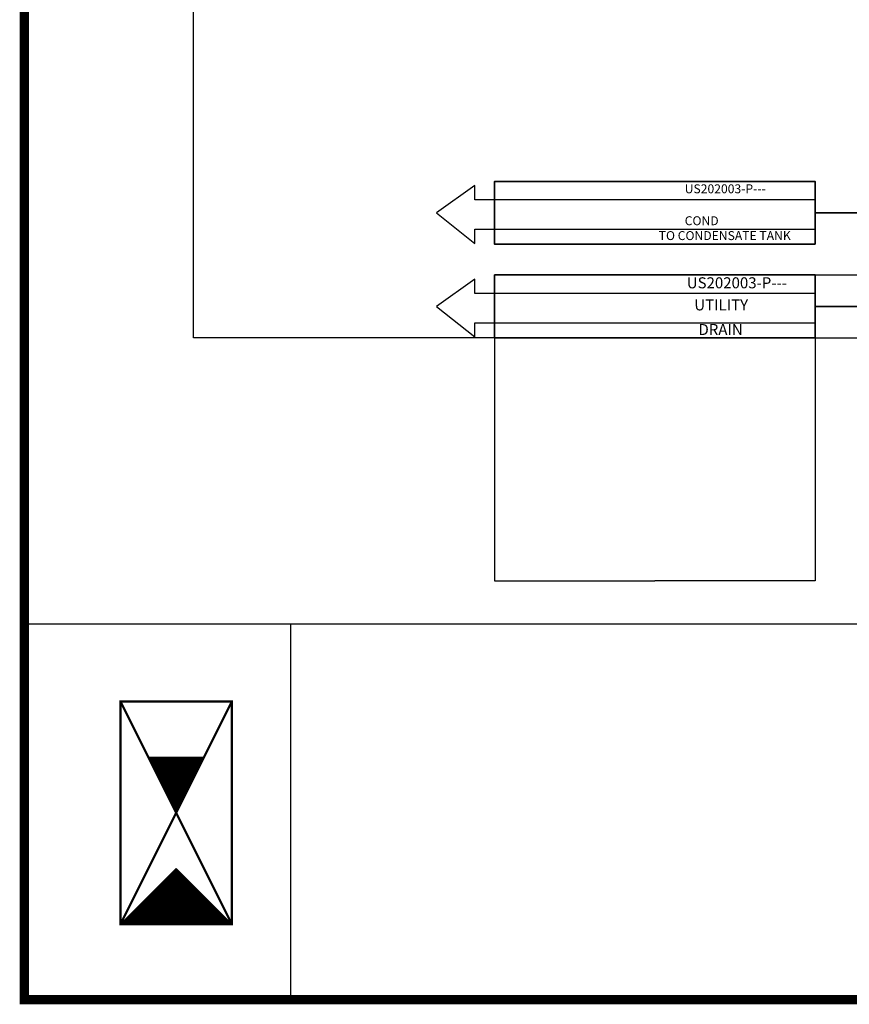
# Model space of a CAD drawing. Units: millimetres. Extents: x 353872 to 441597, y 126154 to 187356.
# Tile 1 of 28: x 353872 to 367541, y 126840 to 143050. Entities that reach past the tile are written whole.
import ezdxf

# ---------------------------------------------------------------- set-up
doc = ezdxf.new("R2010")
doc.units = ezdxf.units.MM
for name, color, linetype, lineweight in [('.', 7, 'Continuous', 0), ('A-ANNO-DIMS', 2, 'Continuous', 18), ('P-ANNO-TEXT', 7, 'Continuous', 25), ('P-ANNO-TTLB', 7, 'Continuous', 25), ('P-EQPM', 5, 'Continuous', 35), ('P-PIPE', 3, 'Continuous', 35)]:
    doc.layers.add(name, color=color, linetype=linetype, lineweight=lineweight)
doc.styles.get("Standard").update_dxf_attribs({"font": 'arial.ttf'})
doc.dimstyles.get("Standard").update_dxf_attribs({"dimtxt": 0.18, "dimasz": 0.18, "dimexe": 0.18, "dimexo": 0.0625, "dimgap": 0.09, "dimtad": 0, "dimtih": 1, "dimtoh": 1, "dimdec": 4, "dimzin": 0, "dimdsep": 46, "dimtxsty": 'Standard', "dimcen": 0.09, "dimadec": 0, "dimazin": 0, "dimtfac": 1, "dimtdec": 4, "dimtofl": 0, "dimtmove": 0, "dimatfit": 3, "dimfxl": 1, "dimtolj": 1, "dimtzin": 0, "dimarcsym": 0})
pattern_1 = [(45, (0, 0), (-0.0883883476483185, 0.0883883476483185), [])]

# ---------------------------------------------------------------- blocks, each defined once
blk = doc.blocks.new('LOGO')
at = {"layer": '.', "ltscale": 0.5}
h = blk.add_hatch(dxfattribs=at)
h.set_pattern_fill('ANSI31', color=256)
h.set_pattern_definition(pattern_1)
h.paths.add_polyline_path([(-25, 50), (0, 0), (25, 50)])
h = blk.add_hatch(dxfattribs=at)
h.set_pattern_fill('ANSI31', color=256)
h.set_pattern_definition(pattern_1)
h.paths.add_polyline_path([(50, -100), (-1.8e-15, -49.99999999906868), (-50, -100)])
at = {"ltscale": 0.5}
blk.add_line((-25, 50), (25, 50), dxfattribs=at)
at = {"ltscale": 0.5, "const_width": 2}
for points in [[(-50, 100), (-50, 100), (0, 0), (50, 100), (50, 100)], [(-50, -100), (-50, -100), (0, 0), (50, -100), (50, -100)]]:
    blk.add_lwpolyline(points, dxfattribs=at)
blk.add_lwpolyline([(-50, 100), (50, 100), (50, -100), (-50, -100)], close=True, dxfattribs=at)
at = {"ltscale": 0.5}
blk.add_lwpolyline([(-50, -100), (0, -49.99999999906868), (50, -100), (-50, -100)], dxfattribs=at)
blk = doc.blocks.new('*D25')
at = {"layer": 'A-ANNO-DIMS', "color": 0, "lineweight": -2, "transparency": 16777216}
for p, q in [((360736.4843020002, 182546.052974), (356736.3668020003, 182546.052974)), ((356736.5468020003, 182545.8729740001), (356736.5468020003, 160179.6269640294)), ((356736.5468020003, 137813.017025), (356736.5468020003, 160179.2630349707)), ((361695.7183060002, 137812.837025), (356736.3668020003, 137812.837025))]:
    blk.add_line(p, q, dxfattribs=at)
at = {"layer": 'A-ANNO-DIMS', "color": 0, "transparency": 16777216}
for points in [[(356736.5168020002, 182545.8729740001), (356736.5768020003, 182545.8729740001), (356736.5468020003, 182546.052974)], [(356736.5168020002, 137813.017025), (356736.5768020003, 137813.017025), (356736.5468020003, 137812.837025)]]:
    blk.add_solid(points, dxfattribs=at)
at = {"layer": 'Defpoints', "color": 0, "transparency": 16777216}
for p in [(360736.5468020002, 182546.052974), (356736.5468020003, 137812.837025), (361695.7808060001, 137812.837025)]:
    blk.add_point(p, dxfattribs=at)
at = {"layer": 'A-ANNO-DIMS', "color": 0, "transparency": 16777216, "insert": (356736.5468020003, 160179.4449994999), "char_height": 0.18, "attachment_point": 5}
blk.add_mtext('\\A1;44733', dxfattribs=at)
blk = doc.blocks.new('*D26')
at = {"layer": 'A-ANNO-DIMS', "color": 0, "lineweight": -2, "transparency": 16777216}
for p, q in [((361695.780806, 137812.774525), (361695.780806, 133812.657025)), ((366976.7551870001, 137812.774525), (366976.7551870001, 133812.657025)), ((361695.960806, 133812.837025), (364335.9265981371, 133812.837025)), ((366976.575187, 133812.837025), (364336.609394863, 133812.837025))]:
    blk.add_line(p, q, dxfattribs=at)
at = {"layer": 'A-ANNO-DIMS', "color": 0, "transparency": 16777216}
for points in [[(361695.960806, 133812.867025), (361695.960806, 133812.807025), (361695.780806, 133812.837025)], [(366976.575187, 133812.867025), (366976.575187, 133812.807025), (366976.7551870001, 133812.837025)]]:
    blk.add_solid(points, dxfattribs=at)
at = {"layer": 'Defpoints', "color": 0, "transparency": 16777216}
for p in [(361695.780806, 137812.837025), (366976.7551870001, 137812.837025), (366976.7551870001, 133812.837025)]:
    blk.add_point(p, dxfattribs=at)
at = {"layer": 'A-ANNO-DIMS', "color": 0, "transparency": 16777216, "insert": (364336.2679965, 133812.837025), "char_height": 0.18, "attachment_point": 5}
blk.add_mtext('\\A1;5281', dxfattribs=at)
blk = doc.blocks.new('*D27')
at = {"layer": 'A-ANNO-DIMS', "color": 0, "lineweight": -2, "transparency": 16777216}
for p, q in [((366976.8176870001, 138848.060561), (440591.1818100004, 138848.060561)), ((440591.0018100004, 138847.8805610001), (440591.0018100004, 138330.6307575294)), ((440591.0018100004, 137813.017025), (440591.0018100004, 138330.2668284707)), ((366976.8176870001, 137812.837025), (440591.1818100004, 137812.837025))]:
    blk.add_line(p, q, dxfattribs=at)
at = {"layer": 'A-ANNO-DIMS', "color": 0, "transparency": 16777216}
for points in [[(440590.9718100004, 138847.8805610001), (440591.0318100004, 138847.8805610001), (440591.0018100004, 138848.060561)], [(440590.9718100004, 137813.017025), (440591.0318100004, 137813.017025), (440591.0018100004, 137812.837025)]]:
    blk.add_solid(points, dxfattribs=at)
at = {"layer": 'Defpoints', "color": 0, "transparency": 16777216}
for p in [(366976.7551870001, 138848.060561), (366976.7551870001, 137812.837025), (440591.0018100004, 137812.837025)]:
    blk.add_point(p, dxfattribs=at)
at = {"layer": 'A-ANNO-DIMS', "color": 0, "transparency": 16777216, "insert": (440591.0018100004, 138330.4487929999), "char_height": 0.18, "attachment_point": 5}
blk.add_mtext('\\A1;1035.2', dxfattribs=at)

msp = doc.modelspace()

# ---------------------------------------------------------------- linework, layer by layer
at = {"layer": 'P-ANNO-TTLB'}
msp.add_line((353948.027365095, 133103.9219526489), (440835.1896390488, 133103.9219526489), dxfattribs=at)
at = {"layer": 'P-ANNO-TTLB', "ltscale": 0.5}
msp.add_line((358335.0178812332, 133103.9219526489), (358335.0178812332, 126916.340154238), dxfattribs=at)
at = {"layer": 'P-ANNO-TTLB', "const_width": 152.4336180244531}
msp.add_lwpolyline([(353948.027365095, 187280.0528919451), (353948.027365095, 126916.340154238), (440835.1896390488, 126916.340154238), (440835.1896390488, 187280.0528919451)], close=True, dxfattribs=at)
at = {"layer": 'P-ANNO-TTLB'}
for points in [[(366976.7551871072, 140084.5530813161), (361369.9490425979, 140084.5530813161), (361369.9490425979, 140318.5333806309), (360736.5468018789, 139870.4641427255), (361369.9490425979, 139367.4195692754), (361369.9490425979, 139601.3998685902), (366976.7551871072, 139601.3998685902)], [(366976.7551871072, 138544.5377317878), (361369.9490425979, 138544.5377317878), (361369.9490425979, 138778.5180311025), (360736.5468018789, 138330.448793197), (361369.9490425979, 137827.4042197469), (361369.9490425979, 138061.3845190617), (366976.7551871072, 138061.3845190617)]]:
    msp.add_lwpolyline(points, dxfattribs=at)
at = {"layer": 'P-EQPM'}
for points in [[(366976.7551871072, 139352.8523745578), (361695.7808057135, 139352.8523745578), (361695.7808057135, 140388.0759108931), (366976.7551871072, 140388.0759108931)], [(366976.7551871072, 137812.8370250294), (361695.7808057135, 137812.8370250294), (361695.7808057135, 138848.0605613646), (366976.7551871072, 138848.0605613646)]]:
    msp.add_lwpolyline(points, close=True, dxfattribs=at)
at = {"layer": 'P-PIPE'}
msp.add_line((366976.7551871072, 138330.448793197), (381521.2667513259, 138330.448793197), dxfattribs=at)
msp.add_lwpolyline([(378690.5041107035, 139870.4641427255), (378361.7180714816, 139870.4641427255, 0.9912181088121462), (378239.2179874769, 139870.4641427255), (366976.7551871072, 139870.4641427255)], format="xyb", dxfattribs=at)

# ---------------------------------------------------------------- block references
at = {"layer": 'P-ANNO-TTLB', "xscale": 18.34344602605143, "yscale": 18.34344602605143, "zscale": 18.34344602605143}
msp.add_blockref('LOGO', (356450.3617875155, 129992.1658918861), dxfattribs=at)

# ---------------------------------------------------------------- texts
at = {"layer": 'P-ANNO-TEXT'}
for s, height, p in [('US202003-P---', 146.8314391480259, (364828.8239641415, 140192.9325025955)), ('COND', 146.8314391480259, (364828.8239641415, 139667.0009499851)), ('TO CONDENSATE TANK', 146.8314391480259, (364400.0555194523, 139422.383555757)), ('US202003-P---', 181.4449954753344, (364862.7502921565, 138627.9607251264)), ('UTILITY', 181.4449954753344, (364986.4498477008, 138263.9798606744)), ('DRAIN', 181.4449954753344, (365055.2991148313, 137859.1053258672))]:
    msp.add_text(s, height=height, dxfattribs=at).set_placement(p)

# ---------------------------------------------------------------- dimensions: what is measured, and where the dimension line sits
at = {"layer": 'A-ANNO-DIMS'}
for base, p1, p2, override, picture, middle in [((356736.5468020003, 137812.837025), (360736.5468020001, 182546.052974), (361695.780806, 137812.837025), {"dimdec": 0, "dimlfac": 1, "dimrnd": 0, "dimzin": 0, "dimdsep": 46, "dimlunit": 2}, '*D25', (356736.5468020003, 160179.4449994999)), ((440591.0018100004, 137812.837025), (366976.7551870001, 138848.060561), (366976.7551870001, 137812.837025), {"dimdec": 1, "dimlfac": 1, "dimrnd": 0, "dimzin": 0, "dimdsep": 46, "dimlunit": 2}, '*D27', (440591.0018100004, 138330.4487929999))]:
    dim = msp.add_linear_dim(base=base, p1=p1, p2=p2, angle=90, dimstyle='Standard', override=override, dxfattribs=at)
    dim.commit()
    dim.dimension.update_dxf_attribs({"geometry": picture, "text_midpoint": middle})
dim = msp.add_linear_dim(base=(366976.7551870001, 133812.837025), p1=(361695.780806, 137812.837025), p2=(366976.7551870001, 137812.837025), dimstyle='Standard', override={"dimdec": 0, "dimlfac": 1, "dimrnd": 0, "dimzin": 0, "dimdsep": 46, "dimlunit": 2}, dxfattribs=at)
dim.commit()
dim.dimension.update_dxf_attribs({"geometry": '*D26', "text_midpoint": (364336.2679965, 133812.837025)})

doc.saveas('drawing.dxf')
